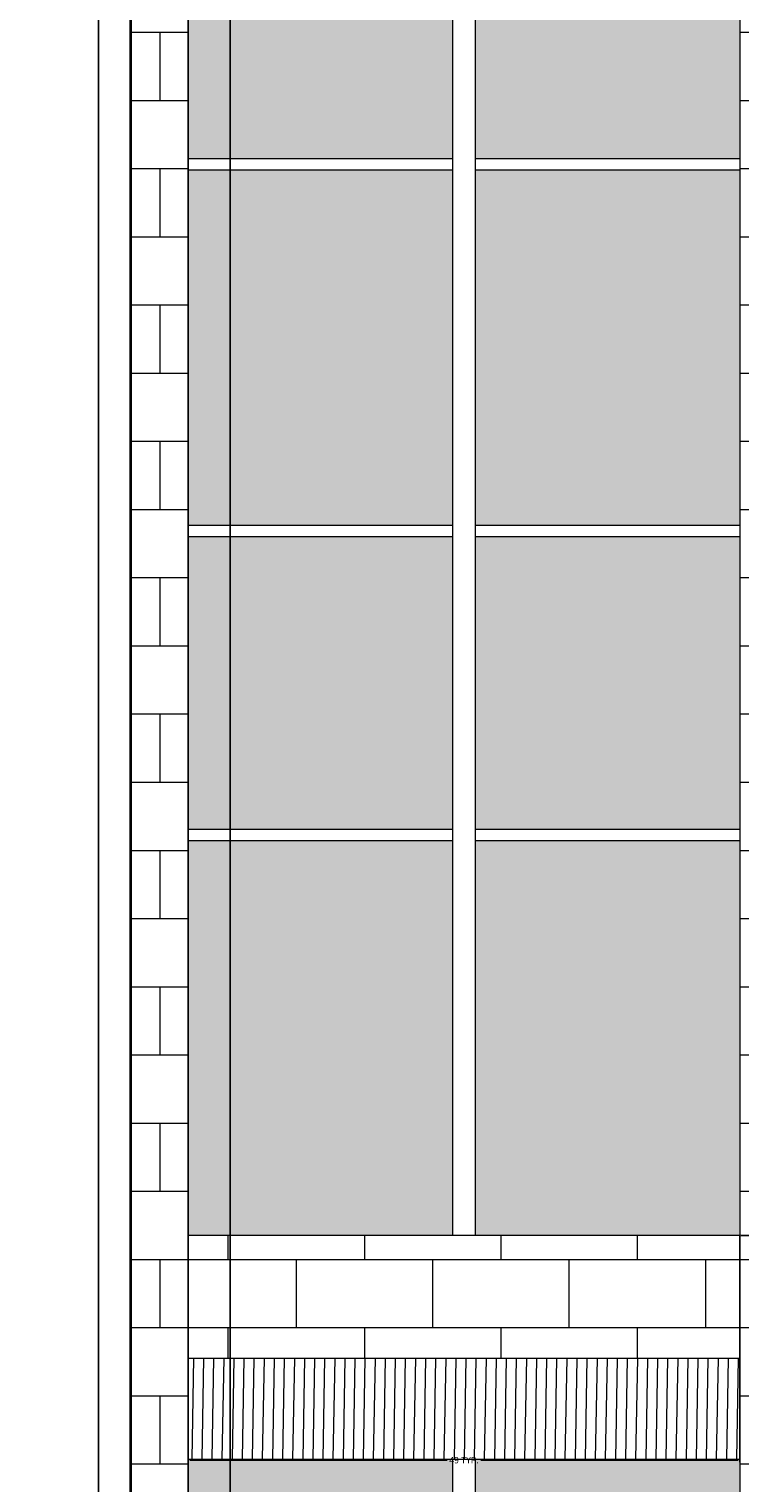
# Model space of a CAD drawing. Units: inches. Extents: x -26 to 776, y -22 to 650.
# Tile 23 of 62: x 222 to 285, y 292 to 420. Entities that reach past the tile are written whole.
import ezdxf

# ---------------------------------------------------------------- set-up
doc = ezdxf.new("R2010")
doc.units = ezdxf.units.IN
doc.header["$MEASUREMENT"] = 0
for name, color, linetype, lineweight in [('A-ANNO-DIMS', 2, 'Continuous', 18), ('A-DETL-PATT', 8, 'Continuous', 13), ('A-GLAZ', 4, 'Continuous', 18), ('A-GLAZ-PATT', 9, 'Continuous', 13), ('A-WALL', 7, 'Continuous', 35), ('A-WALL-PATT', 8, 'Continuous', 13)]:
    doc.layers.add(name, color=color, linetype=linetype, lineweight=lineweight)
doc.styles.get("Standard").update_dxf_attribs({"font": 'arial.ttf'})
doc.dimstyles.get("Standard").update_dxf_attribs({"dimtxt": 0.5625, "dimasz": 0.18, "dimexe": 0.18, "dimexo": 0.0625, "dimgap": 0.09, "dimtad": 0, "dimtih": 1, "dimtoh": 1, "dimdec": 4, "dimzin": 0, "dimdsep": 46, "dimlunit": 4, "dimtxsty": 'Standard', "dimcen": 0.09, "dimadec": 0, "dimazin": 0, "dimtfac": 1, "dimtdec": 4, "dimtofl": 0, "dimtmove": 0, "dimatfit": 3, "dimfxl": 1, "dimtolj": 1, "dimtzin": 0, "dimarcsym": 0})

# ---------------------------------------------------------------- blocks, each defined once
blk = doc.blocks.new('WIN-ELEV-2X4-HEAD')
for p, q in [((0, 123), (0, 131.89)), ((0, 131.89), (48.55, 131.89)), ((48.55, 131.89), (48.55, 123)), ((23.28, 0), (23.28, 123)), ((25.28, 0), (25.28, 123)), ((0, 94.77), (23.28, 94.77)), ((25.28, 94.77), (48.55, 94.77)), ((0, 93.77), (23.28, 93.77)), ((25.28, 93.77), (48.55, 93.77)), ((0, 62.5), (23.28, 62.5)), ((0, 61.5), (23.28, 61.5)), ((25.28, 62.5), (48.55, 62.5)), ((25.28, 61.5), (48.55, 61.5)), ((0, 35.76), (23.28, 35.76)), ((0, 34.76), (23.28, 34.76)), ((25.28, 35.76), (48.55, 35.76)), ((25.28, 34.76), (48.55, 34.76))]:
    blk.add_line(p, q)
blk.add_lwpolyline([(48.55, 0), (0, 0), (0, 123), (48.55, 123)], close=True)
blk = doc.blocks.new('*D9')
at = {"layer": 'A-ANNO-DIMS', "color": 0, "lineweight": -2, "transparency": 16777216}
for p, q in [((285.08, 446.01), (304.98, 446.01)), ((304.8, 445.83), (304.8, 380.44)), ((304.8, 314.3), (304.8, 379.68)), ((285.08, 314.12), (304.98, 314.12))]:
    blk.add_line(p, q, dxfattribs=at)
at = {"layer": 'A-ANNO-DIMS', "color": 0, "transparency": 16777216}
for points in [[(304.77, 445.83), (304.83, 445.83), (304.8, 446.01)], [(304.77, 314.3), (304.83, 314.3), (304.8, 314.12)]]:
    blk.add_solid(points, dxfattribs=at)
at = {"layer": 'Defpoints', "color": 0, "transparency": 16777216}
for p in [(285.02, 446.01), (304.8, 446.01), (285.02, 314.12)]:
    blk.add_point(p, dxfattribs=at)
at = {"layer": 'A-ANNO-DIMS', "color": 0, "transparency": 16777216, "insert": (304.8, 380.06), "char_height": 0.5625, "attachment_point": 5}
blk.add_mtext('\\A1;NARROW WINDOW 132 TYP.', dxfattribs=at)
blk = doc.blocks.new('*D10')
at = {"layer": 'A-ANNO-DIMS', "color": 0, "lineweight": -2, "transparency": 16777216}
for p, q in [((236.46, 314.06), (236.46, 294.16)), ((285.02, 314.06), (285.02, 294.16)), ((236.64, 294.34), (259.27, 294.34)), ((284.84, 294.34), (262.21, 294.34))]:
    blk.add_line(p, q, dxfattribs=at)
at = {"layer": 'A-ANNO-DIMS', "color": 0, "transparency": 16777216}
for points in [[(236.64, 294.37), (236.64, 294.31), (236.46, 294.34)], [(284.84, 294.37), (284.84, 294.31), (285.02, 294.34)]]:
    blk.add_solid(points, dxfattribs=at)
at = {"layer": 'Defpoints', "color": 0, "transparency": 16777216}
for p in [(236.46, 314.12), (285.02, 314.12), (285.02, 294.34)]:
    blk.add_point(p, dxfattribs=at)
at = {"layer": 'A-ANNO-DIMS', "color": 0, "transparency": 16777216, "insert": (260.74, 294.34), "char_height": 0.5625, "attachment_point": 5}
blk.add_mtext('\\A1;49 TYP.', dxfattribs=at)
blk = doc.blocks.new('*D34')
at = {"layer": 'A-ANNO-DIMS', "color": 0, "lineweight": -2, "transparency": 16777216}
for p, q in [((228.57, 528.3), (228.57, -21.31)), ((357.3, 528.36), (357.3, -21.31)), ((228.75, -21.13), (291.71, -21.13)), ((357.12, -21.13), (294.17, -21.13))]:
    blk.add_line(p, q, dxfattribs=at)
at = {"layer": 'A-ANNO-DIMS', "color": 0, "transparency": 16777216}
for points in [[(228.75, -21.1), (228.75, -21.16), (228.57, -21.13)], [(357.12, -21.1), (357.12, -21.16), (357.3, -21.13)]]:
    blk.add_solid(points, dxfattribs=at)
at = {"layer": 'Defpoints', "color": 0, "transparency": 16777216}
for p in [(357.3, 528.42), (228.57, 528.36), (357.3, -21.13)]:
    blk.add_point(p, dxfattribs=at)
at = {"layer": 'A-ANNO-DIMS', "color": 0, "transparency": 16777216, "insert": (292.94, -21.13), "char_height": 0.562, "attachment_point": 5}
blk.add_mtext('\\A1;128.73', dxfattribs=at)
blk = doc.blocks.new('*D43')
at = {"layer": 'A-ANNO-DIMS', "color": 0, "lineweight": -2, "transparency": 16777216}
for p, q in [((231.42, 159.54), (231.42, 649.86)), ((231.6, 649.68), (233.13, 649.68)), ((236.28, 649.68), (234.76, 649.68)), ((236.46, 171.48), (236.46, 649.86))]:
    blk.add_line(p, q, dxfattribs=at)
at = {"layer": 'A-ANNO-DIMS', "color": 0, "transparency": 16777216}
for points in [[(231.6, 649.71), (231.6, 649.65), (231.42, 649.68)], [(236.28, 649.71), (236.28, 649.65), (236.46, 649.68)]]:
    blk.add_solid(points, dxfattribs=at)
at = {"layer": 'Defpoints', "color": 0, "transparency": 16777216}
for p in [(236.46, 649.68), (236.46, 171.42), (231.42, 159.48)]:
    blk.add_point(p, dxfattribs=at)
at = {"layer": 'A-ANNO-DIMS', "color": 0, "transparency": 16777216, "insert": (233.94, 649.68), "char_height": 0.562, "attachment_point": 5}
blk.add_mtext('\\A1;5.04', dxfattribs=at)
blk = doc.blocks.new('*D44')
at = {"layer": 'A-ANNO-DIMS', "color": 0, "lineweight": -2, "transparency": 16777216}
for p, q in [((231.42, 15.54), (231.42, 649.86)), ((231.6, 649.68), (234.98, 649.68)), ((239.99, 649.68), (236.61, 649.68)), ((240.17, 26.49), (240.17, 649.86))]:
    blk.add_line(p, q, dxfattribs=at)
at = {"layer": 'A-ANNO-DIMS', "color": 0, "transparency": 16777216}
for points in [[(231.6, 649.71), (231.6, 649.65), (231.42, 649.68)], [(239.99, 649.71), (239.99, 649.65), (240.17, 649.68)]]:
    blk.add_solid(points, dxfattribs=at)
at = {"layer": 'Defpoints', "color": 0, "transparency": 16777216}
for p in [(240.17, 649.68), (240.17, 26.42), (231.42, 15.48)]:
    blk.add_point(p, dxfattribs=at)
at = {"layer": 'A-ANNO-DIMS', "color": 0, "transparency": 16777216, "insert": (235.8, 649.68), "char_height": 0.562, "attachment_point": 5}
blk.add_mtext('\\A1;8.74', dxfattribs=at)

msp = doc.modelspace()

# ---------------------------------------------------------------- hatches: boundary and pattern name
at = {"layer": 'A-DETL-PATT'}
h = msp.add_hatch(dxfattribs=at)
h.set_pattern_fill('ANSI31', color=256, scale=7.1, angle=44)
h.paths.add_polyline_path([(231.4249, 197.3298), (216.1056, 197.3298), (216.1056, 159.4824), (231.4249, 159.4824)])
h.paths.add_polyline_path([(236.4647, 197.3298), (231.4249, 197.3298), (231.4249, 159.4824), (276.1134, 159.4824), (276.1134, 171.4173), (236.4647, 171.4173)])
h.paths.add_polyline_path([(259.7413, 197.3298), (236.4647, 197.3298), (236.4647, 171.4173), (259.7413, 171.4173)], flags=17)
h.paths.add_polyline_path([(276.1134, 197.3298), (261.7413, 197.3298), (261.7413, 171.4173), (276.1134, 171.4173)], flags=17)
h.paths.add_polyline_path([(217.9529, 147.0781), (22.8891, 147.0781), (22.8891, 138.3844), (217.9529, 138.3844)])
h.paths.add_polyline_path([(285.0179, 152.3087), (285.0179, 159.4824), (231.4249, 159.4824), (240.1654, 144.8359), (280.6173, 144.8359)])
h.paths.add_polyline_path([(280.6173, 144.8359), (240.1654, 144.8359), (240.1654, 26.4239), (280.6173, 26.4239)])
h.paths.add_polyline_path([(274.6644, 134.8811), (274.6644, 34.0885), (245.7207, 34.0885), (245.7207, 134.8811)], flags=16)
h.paths.add_polyline_path([(285.0179, 303.3046), (236.4647, 303.3046), (236.4647, 294.4171), (285.0179, 294.4171)])
h.paths.add_polyline_path([(285.0179, 446.0063), (236.4647, 446.0063), (236.4647, 437.1188), (285.0179, 437.1188)])
at = {"layer": 'A-GLAZ-PATT'}
h = msp.add_hatch(dxfattribs=at)
h.set_pattern_fill('GOST_GLASS', color=256, scale=0.75)
h.set_pattern_definition([(45, (0, 0), (6.36396, 0), [3.75, -5.25]), (45, (1.591, 0), (6.36396, 0), [1.5, -7.5]), (45, (0, 1.591), (6.36396, 0), [1.5, -7.5])])
h.paths.add_polyline_path([(115.8402, 198.8773), (93.6448, 198.8773), (93.6448, 173.9734), (115.8402, 173.9734)])
h.paths.add_polyline_path([(144.1571, 198.8773), (115.8402, 198.8773), (115.8402, 173.9734), (144.1571, 173.9734)])
h.paths.add_polyline_path([(115.8402, 224.3396), (93.6448, 224.3396), (93.6448, 198.8773), (115.8402, 198.8773)])
h.paths.add_polyline_path([(144.1571, 248.4417), (115.8402, 248.4417), (115.8402, 224.3396), (144.1571, 224.3396)])
h.paths.add_polyline_path([(144.1571, 224.3396), (115.8402, 224.3396), (115.8402, 198.8773), (144.1571, 198.8773)])
h.paths.add_polyline_path([(170.5449, 224.3396), (144.1571, 224.3396), (144.1571, 198.8773), (170.5449, 198.8773)])
h.paths.add_polyline_path([(170.5449, 198.8773), (144.1571, 198.8773), (144.1571, 173.9734), (170.5449, 173.9734)])
h.paths.add_polyline_path([(194.6694, 198.8773), (170.5449, 198.8773), (170.5449, 173.9734), (194.6694, 173.9734)])
h.paths.add_polyline_path([(194.6694, 224.3396), (170.5449, 224.3396), (170.5449, 198.8773), (194.6694, 198.8773)])
h.paths.add_polyline_path([(194.6694, 248.4417), (170.5449, 248.4417), (170.5449, 224.3396), (194.6694, 224.3396)])
h.paths.add_polyline_path([(170.5449, 248.4417), (144.1571, 248.4417), (144.1571, 224.3396), (170.5449, 224.3396)])
h.paths.add_polyline_path([(144.1571, 269.3091), (115.8402, 269.3091), (115.8402, 248.4417), (144.1571, 248.4417)])
h.paths.add_polyline_path([(115.8402, 269.3091), (93.6448, 269.3091), (93.6448, 248.4417), (115.8402, 248.4417)])
h.paths.add_polyline_path([(115.8402, 248.4417), (93.6448, 248.4417), (93.6448, 224.3396), (115.8402, 224.3396)])
h.paths.add_polyline_path([(170.5449, 269.3091), (144.1571, 269.3091), (144.1571, 248.4417), (170.5449, 248.4417)])
h.paths.add_polyline_path([(194.6694, 269.3091), (170.5449, 269.3091), (170.5449, 248.4417), (194.6694, 248.4417)])
h.paths.add_polyline_path([(259.7413, 294.4171), (236.4647, 294.4171), (236.4647, 266.1888), (259.7413, 266.1888)])
h.paths.add_polyline_path([(285.0179, 294.4171), (261.7413, 294.4171), (261.7413, 266.1888), (285.0179, 266.1888)])
h.paths.add_polyline_path([(285.0179, 265.1888), (261.7413, 265.1888), (261.7413, 233.9172), (285.0179, 233.9172)])
h.paths.add_polyline_path([(259.7413, 265.1888), (236.4647, 265.1888), (236.4647, 233.9172), (259.7413, 233.9172)])
h.paths.add_polyline_path([(259.7413, 232.9172), (236.4647, 232.9172), (236.4647, 207.1741), (259.7413, 207.1741)])
h.paths.add_polyline_path([(285.0179, 232.9172), (261.7413, 232.9172), (261.7413, 207.1741), (285.0179, 207.1741)])
h.paths.add_polyline_path([(285.0179, 206.1741), (261.7413, 206.1741), (261.7413, 199.3298), (278.1134, 199.3298), (278.1134, 171.4173), (285.0179, 171.4173)])
h.paths.add_polyline_path([(259.7413, 206.1741), (236.4647, 206.1741), (236.4647, 199.3298), (259.7413, 199.3298)])
h.paths.add_polyline_path([(259.7413, 197.3298), (236.4647, 197.3298), (236.4647, 171.4173), (259.7413, 171.4173)])
h.paths.add_polyline_path([(276.1134, 197.3298), (261.7413, 197.3298), (261.7413, 171.4173), (276.1134, 171.4173)], flags=17)
h.paths.add_polyline_path([(255.8125, 548.0348), (228.5733, 548.0348), (228.5733, 528.3585), (255.8125, 528.3585)])
h.paths.add_polyline_path([(281.6181, 548.0348), (256.0792, 548.0348), (256.0792, 528.3585), (281.6181, 528.3585)])
h.paths.add_polyline_path([(308.8797, 548.0348), (281.789, 548.0348), (281.789, 528.3585), (308.8797, 528.3585)])
h.paths.add_polyline_path([(357.2724, 548.0995), (309.2457, 548.0348), (309.2457, 528.3585), (357.3034, 528.4233), (357.3034, 538.2614)])
h.paths.add_polyline_path([(259.7413, 437.1188), (236.4647, 437.1188), (236.4647, 408.8905), (259.7413, 408.8905)])
h.paths.add_polyline_path([(285.0179, 437.1188), (261.7413, 437.1188), (261.7413, 408.8905), (285.0179, 408.8905)])
h.paths.add_polyline_path([(259.7413, 407.8905), (236.4647, 407.8905), (236.4647, 376.6189), (259.7413, 376.6189)])
h.paths.add_polyline_path([(285.0179, 407.8905), (261.7413, 407.8905), (261.7413, 376.6189), (285.0179, 376.6189)])
h.paths.add_polyline_path([(285.0179, 375.6189), (261.7413, 375.6189), (261.7413, 349.8758), (285.0179, 349.8758)])
h.paths.add_polyline_path([(285.0179, 348.8758), (261.7413, 348.8758), (261.7413, 314.119), (285.0179, 314.119)])
h.paths.add_polyline_path([(259.7413, 348.8758), (236.4647, 348.8758), (236.4647, 314.119), (259.7413, 314.119)])
h.paths.add_polyline_path([(259.7413, 375.6189), (236.4647, 375.6189), (236.4647, 349.8758), (259.7413, 349.8758)])
h.paths.add_polyline_path([(194.6694, 404.1909), (170.5449, 404.1909), (170.5449, 383.3235), (194.6694, 383.3235)])
h.paths.add_polyline_path([(170.5449, 404.1909), (144.1571, 404.1909), (144.1571, 383.3235), (170.5449, 383.3235)])
h.paths.add_polyline_path([(144.1571, 404.1909), (115.8402, 404.1909), (115.8402, 383.3235), (144.1571, 383.3235)])
h.paths.add_polyline_path([(115.8402, 404.1909), (93.6448, 404.1909), (93.6448, 383.3235), (115.8402, 383.3235)])
h.paths.add_polyline_path([(115.8402, 383.3235), (93.6448, 383.3235), (93.6448, 359.2214), (115.8402, 359.2214)])
h.paths.add_polyline_path([(144.1571, 383.3235), (115.8402, 383.3235), (115.8402, 359.2214), (144.1571, 359.2214)])
h.paths.add_polyline_path([(115.8402, 359.2214), (93.6448, 359.2214), (93.6448, 333.7591), (115.8402, 333.7591)])
h.paths.add_polyline_path([(144.1571, 359.2214), (115.8402, 359.2214), (115.8402, 333.7591), (144.1571, 333.7591)])
h.paths.add_polyline_path([(115.8402, 333.7591), (93.6448, 333.7591), (93.6448, 308.8552), (115.8402, 308.8552)])
h.paths.add_polyline_path([(144.1571, 333.7591), (115.8402, 333.7591), (115.8402, 308.8552), (144.1571, 308.8552)])
h.paths.add_polyline_path([(170.5449, 333.7591), (144.1571, 333.7591), (144.1571, 308.8552), (170.5449, 308.8552)])
h.paths.add_polyline_path([(170.5449, 359.2214), (144.1571, 359.2214), (144.1571, 333.7591), (170.5449, 333.7591)])
h.paths.add_polyline_path([(170.5449, 383.3235), (144.1571, 383.3235), (144.1571, 359.2214), (170.5449, 359.2214)])
h.paths.add_polyline_path([(194.6694, 383.3235), (170.5449, 383.3235), (170.5449, 359.2214), (194.6694, 359.2214)])
h.paths.add_polyline_path([(194.6694, 359.2214), (170.5449, 359.2214), (170.5449, 333.7591), (194.6694, 333.7591)])
h.paths.add_polyline_path([(194.6694, 333.7591), (170.5449, 333.7591), (170.5449, 308.8552), (194.6694, 308.8552)])
at = {"layer": 'A-WALL-PATT'}
h = msp.add_hatch(dxfattribs=at)
h.set_pattern_fill('AR-B816', color=256, scale=0.75)
h.paths.add_polyline_path([(289.2424, 504.4205), (231.4249, 504.4205), (231.4249, 458.1203), (231.4249, 221.6413), (231.4249, 209.6413), (231.4249, 159.4824), (285.0179, 159.4824), (285.0179, 171.4173), (236.4647, 171.4173), (236.4647, 294.4171), (236.4647, 303.3046), (285.0179, 303.3046), (285.0179, 294.4171), (285.0179, 171.4173), (285.0179, 159.4824), (289.2424, 159.4824), (289.2424, 291.1798), (289.2424, 458.1203)])
h.paths.add_polyline_path([(285.0179, 446.0063), (285.0179, 437.1188), (285.0179, 314.119), (236.4647, 314.119), (236.4647, 437.1188), (236.4647, 446.0063)], flags=16)

# ---------------------------------------------------------------- linework, layer by layer
at = {"layer": 'A-WALL'}
msp.add_line((231.4249, 221.6413), (231.4249, 458.1203), dxfattribs=at)

# ---------------------------------------------------------------- block references
at = {"layer": 'A-GLAZ'}
for p in [(236.465, 314.1187), (236.465, 171.417)]:
    msp.add_blockref('WIN-ELEV-2X4-HEAD', p, dxfattribs=at)

# ---------------------------------------------------------------- dimensions: what is measured, and where the dimension line sits
at = {"layer": 'A-ANNO-DIMS'}
for base, p1, p2, picture, middle in [((236.4647, 649.6763), (231.4249, 159.4824), (236.4647, 171.4173), '*D43', (233.9448, 649.6763)), ((240.1654, 649.6763), (231.4249, 15.4824), (240.1654, 26.4239), '*D44', (235.7952, 649.6763)), ((357.3034, -21.1349), (228.5733, 528.3585), (357.3034, 528.4233), '*D34', (292.9384, -21.1349))]:
    dim = msp.add_linear_dim(base=base, p1=p1, p2=p2, dimstyle='Standard', override={"dimdec": 2, "dimlfac": 1, "dimrnd": 0, "dimzin": 0, "dimdsep": 46, "dimlunit": 2}, dxfattribs=at)
    dim.commit()
    dim.dimension.update_dxf_attribs({"geometry": picture, "text_midpoint": middle})
dim = msp.add_linear_dim(base=(304.801, 446.0063), p1=(285.0179, 314.119), p2=(285.0179, 446.0063), angle=90, text='NARROW WINDOW <> TYP.', dimstyle='Standard', override={"dimdec": 0, "dimlfac": 1, "dimrnd": 0, "dimzin": 0, "dimdsep": 46, "dimlunit": 2}, dxfattribs=at)
dim.commit()
dim.dimension.update_dxf_attribs({"geometry": '*D9', "text_midpoint": (304.801, 380.0626)})
dim = msp.add_linear_dim(base=(285.0179, 294.3359), p1=(236.4647, 314.119), p2=(285.0179, 314.119), text='<> TYP.', dimstyle='Standard', override={"dimdec": 0, "dimlfac": 1, "dimrnd": 0, "dimzin": 0, "dimdsep": 46, "dimlunit": 2}, dxfattribs=at)
dim.commit()
dim.dimension.update_dxf_attribs({"geometry": '*D10', "text_midpoint": (260.7413, 294.3359)})

doc.saveas('drawing.dxf')
